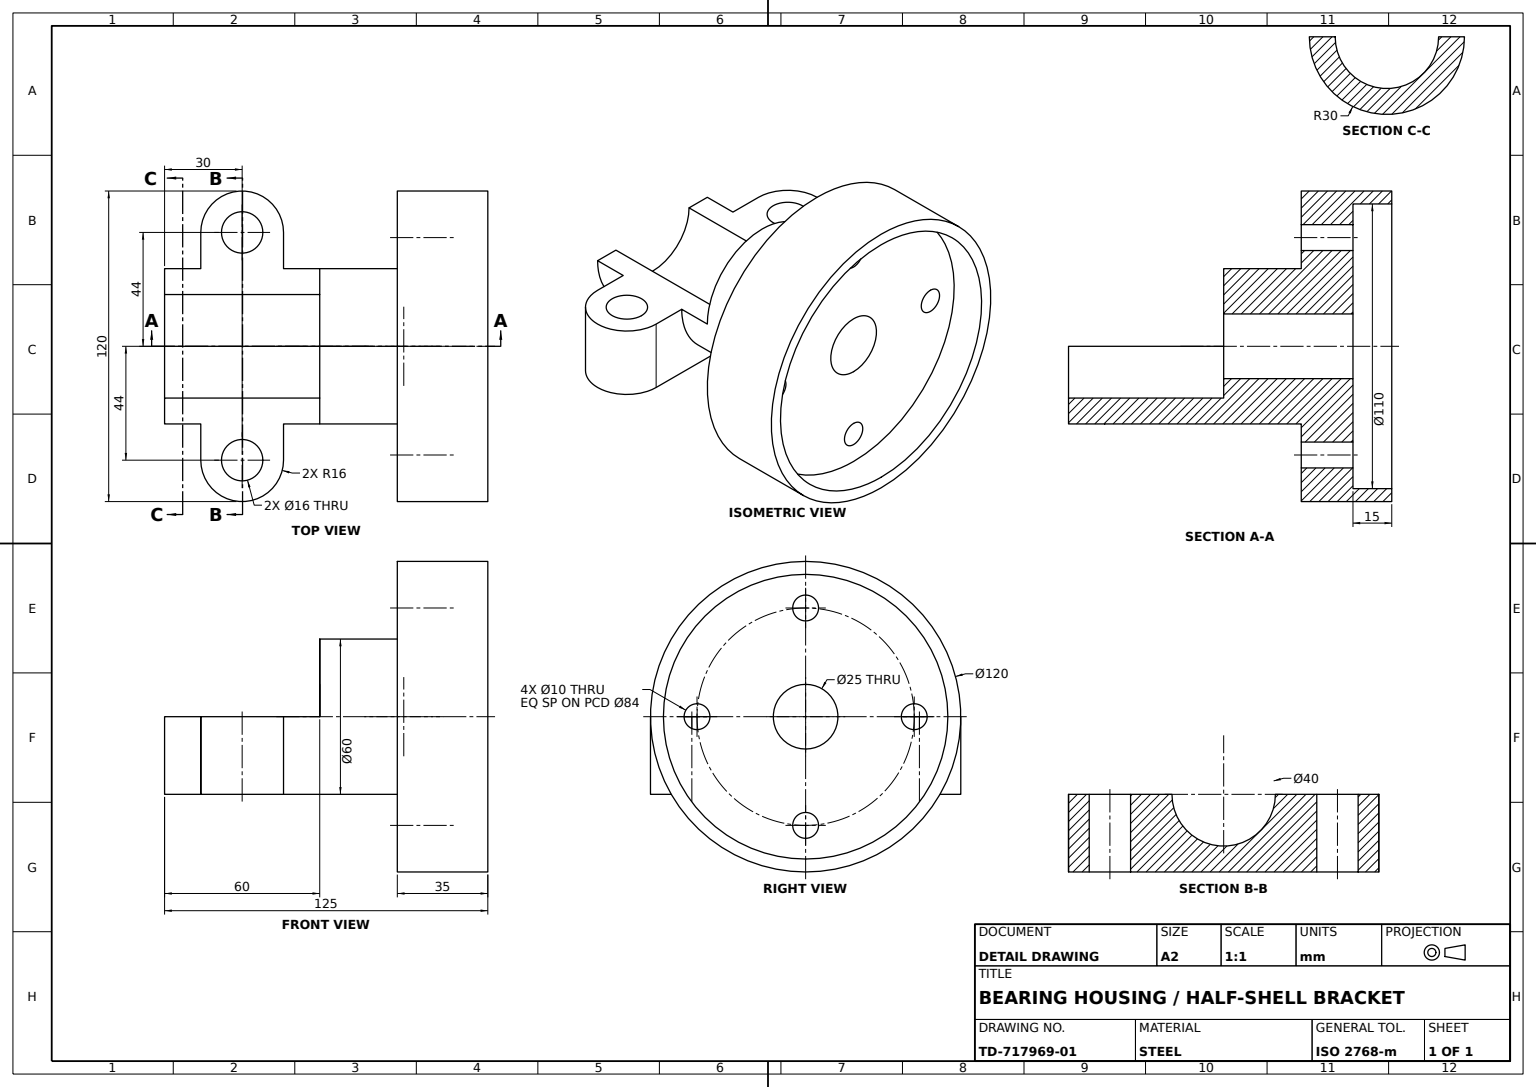
from build123d import *

# Parameters (mm, degrees)
FLANGE_BOLT_HOLES_4X_10_REACH = 93.788
FLANGE_BOLT_HOLES_SKETCH_R    = 5
BEARING_START                 = 60
BEARING_BLOCK_DEPTH           = 60
SPLIT_CAP_LUGS_SKETCH_R       = 8
SPLIT_CAP_LUGS_DEPTH          = 30
JOURNAL_SEAT_SPLIT_CUT_REACH  = 141.718


with BuildPart() as part:
    # Flanged Hub Profile → Flanged Hub (revolve)
    with BuildSketch(Plane.XY):
        Polygon((0, 60), (-35, 60), (-35, 30), (-65, 30), (-65, 12.5), (-15, 12.5), (-15, 55), (0, 55), align=None)
    revolve(axis=Axis((0, 0, 0), (-1, 0, 0)))

    # Flange Bolt Holes Sketch → Flange Bolt Holes 4xØ10 (cut, up to next)
    with BuildSketch(Plane.ZY.offset(35), mode=Mode.PRIVATE) as flange_bolt_holes_4x_10_sk1:
        with Locations(Location((42, 0, 0), (0, 0, 270))):
            Circle(FLANGE_BOLT_HOLES_SKETCH_R)
    flange_bolt_holes_4x_10_tool1 = extrude(flange_bolt_holes_4x_10_sk1.sketch, amount=-FLANGE_BOLT_HOLES_4X_10_REACH, mode=Mode.PRIVATE) & part.part
    # Flange Bolt Holes Sketch → Flange Bolt Holes 4xØ10 (cut, up to next)
    with BuildSketch(Plane.ZY.offset(35), mode=Mode.PRIVATE) as flange_bolt_holes_4x_10_sk2:
        with Locations(Location((0, -42, 0), (0, 0, 270))):
            Circle(FLANGE_BOLT_HOLES_SKETCH_R)
    flange_bolt_holes_4x_10_tool2 = extrude(flange_bolt_holes_4x_10_sk2.sketch, amount=-FLANGE_BOLT_HOLES_4X_10_REACH, mode=Mode.PRIVATE) & part.part
    # Flange Bolt Holes Sketch → Flange Bolt Holes 4xØ10 (cut, up to next)
    with BuildSketch(Plane.ZY.offset(35), mode=Mode.PRIVATE) as flange_bolt_holes_4x_10_sk3:
        with Locations(Location((-42, 0, 0), (0, 0, 270))):
            Circle(FLANGE_BOLT_HOLES_SKETCH_R)
    flange_bolt_holes_4x_10_tool3 = extrude(flange_bolt_holes_4x_10_sk3.sketch, amount=-FLANGE_BOLT_HOLES_4X_10_REACH, mode=Mode.PRIVATE) & part.part
    # Flange Bolt Holes Sketch → Flange Bolt Holes 4xØ10 (cut, up to next)
    with BuildSketch(Plane.ZY.offset(35), mode=Mode.PRIVATE) as flange_bolt_holes_4x_10_sk4:
        with Locations(Location((0, 42, 0), (0, 0, 270))):
            Circle(FLANGE_BOLT_HOLES_SKETCH_R)
    flange_bolt_holes_4x_10_tool4 = extrude(flange_bolt_holes_4x_10_sk4.sketch, amount=-FLANGE_BOLT_HOLES_4X_10_REACH, mode=Mode.PRIVATE) & part.part
    add(flange_bolt_holes_4x_10_tool1.solids().sort_by_distance((-35, 0, 42))[0], mode=Mode.SUBTRACT)
    add(flange_bolt_holes_4x_10_tool2.solids().sort_by_distance((-35, -42, 0))[0], mode=Mode.SUBTRACT)
    add(flange_bolt_holes_4x_10_tool3.solids().sort_by_distance((-35, 0, -42))[0], mode=Mode.SUBTRACT)
    add(flange_bolt_holes_4x_10_tool4.solids().sort_by_distance((-35, 42, 0))[0], mode=Mode.SUBTRACT)

    # Bearing Block Sketch → Bearing Block (add)
    with BuildSketch(Plane.ZY.offset(65).offset(BEARING_START)):
        with BuildLine():
            Line((-30, 0), (-20, 0))
            ThreePointArc((-20, 0), (0, -20), (20, 0))
            Line((20, 0), (30, 0))
            ThreePointArc((30, 0), (0, -30), (-30, 0))
        make_face()
    extrude(amount=-BEARING_BLOCK_DEPTH)

    # Split Cap Lugs Sketch → Split Cap Lugs (add)
    with BuildSketch(Plane(origin=(0, 0, 0), x_dir=(1, 0, 0), z_dir=(0, 1, 0))):
        with BuildLine():
            Line((-111, -44), (-111, 44))
            ThreePointArc((-111, 44), (-95, 60), (-79, 44))
            Line((-79, 44), (-79, -44))
            ThreePointArc((-79, -44), (-95, -60), (-111, -44))
        make_face()
        with Locations(Location((-95, 44, 0), (0, 0, 180))):
            Circle(SPLIT_CAP_LUGS_SKETCH_R, mode=Mode.SUBTRACT)
        with Locations(Location((-95, -44, 0), (0, 0, 180))):
            Circle(SPLIT_CAP_LUGS_SKETCH_R, mode=Mode.SUBTRACT)
    extrude(amount=-SPLIT_CAP_LUGS_DEPTH)

    # Journal Seat Split Sketch → Journal Seat Split Cut (cut, up to next)
    with BuildSketch(Plane.ZY.offset(111), mode=Mode.PRIVATE) as journal_seat_split_cut_sk1:
        with BuildLine():
            Line((20, 0), (-20, 0))
            ThreePointArc((-20, 0), (0, -20), (20, 0))
        make_face()
    journal_seat_split_cut_tool1 = extrude(journal_seat_split_cut_sk1.sketch, amount=-JOURNAL_SEAT_SPLIT_CUT_REACH, mode=Mode.PRIVATE) & part.part
    add(journal_seat_split_cut_tool1.solids().sort_by_distance((-111, -8.488264, 0))[0], mode=Mode.SUBTRACT)


solid = part.part
